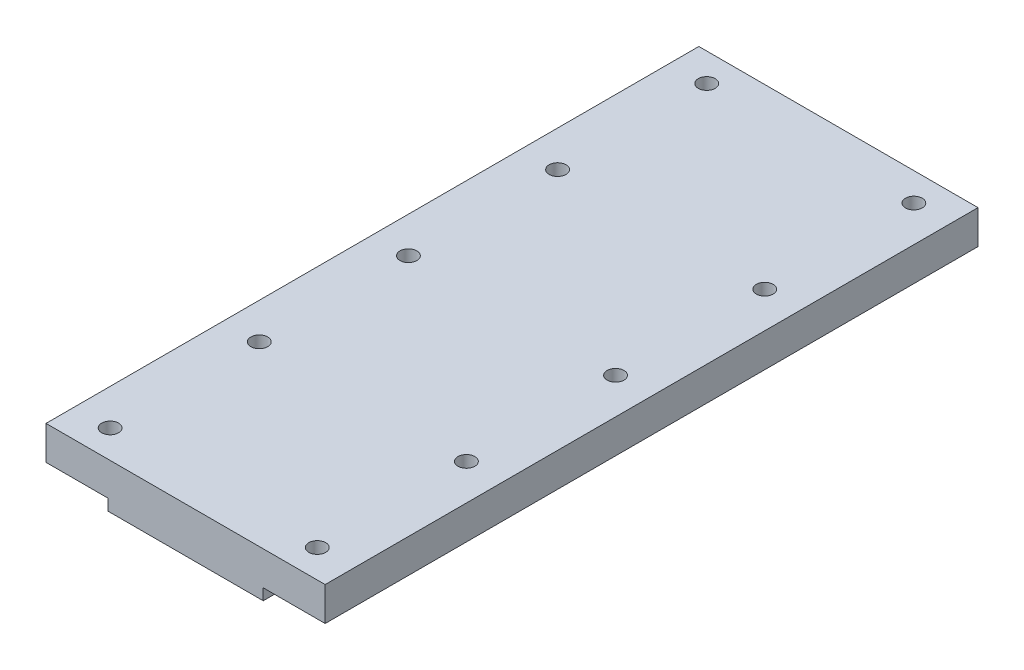
from build123d import *

# Parameters (mm, degrees)
BASE_PLATE_DEPTH            = 290
MOUNTING_HOLES_SKETCH_R     = 7.5
MOUNTING_HOLES_10X_15_DEPTH = 290


with BuildPart() as part:
    # Plate Profile Sketch → Base Plate (new, symmetric)
    with BuildSketch(Plane.XY):
        Polygon((-124, 0), (-69, 0), (-69, -10), (69, -10), (69, 0), (124, 0), (124, 30), (-124, 30), align=None)
    extrude(amount=BASE_PLATE_DEPTH, both=True)

    # Mounting Holes Sketch → Mounting Holes 10xØ15 (cut, symmetric)
    with BuildSketch(Plane(origin=(0, 30, 0), x_dir=(1, 0, 0), z_dir=(0, 1, 0))):
        with Locations(Location((-92, 265, 0), (0, 0, 180))):
            Circle(MOUNTING_HOLES_SKETCH_R)
        with Locations(Location((-92, 132.5, 0), (0, 0, 180))):
            Circle(MOUNTING_HOLES_SKETCH_R)
        with Locations(Location((-92, 0, 0), (0, 0, 180))):
            Circle(MOUNTING_HOLES_SKETCH_R)
        with Locations(Location((-92, -132.5, 0), (0, 0, 180))):
            Circle(MOUNTING_HOLES_SKETCH_R)
        with Locations(Location((-92, -265, 0), (0, 0, 180))):
            Circle(MOUNTING_HOLES_SKETCH_R)
        with Locations(Location((92, 132.5, 0), (0, 0, 270))):
            Circle(MOUNTING_HOLES_SKETCH_R)
        with Locations(Location((92, 0, 0), (0, 0, 270))):
            Circle(MOUNTING_HOLES_SKETCH_R)
        with Locations(Location((92, -132.5, 0), (0, 0, 270))):
            Circle(MOUNTING_HOLES_SKETCH_R)
        with Locations(Location((92, -265, 0), (0, 0, 270))):
            Circle(MOUNTING_HOLES_SKETCH_R)
        with Locations(Location((92, 265, 0), (0, 0, 270))):
            Circle(MOUNTING_HOLES_SKETCH_R)
    extrude(amount=MOUNTING_HOLES_10X_15_DEPTH, both=True, mode=Mode.SUBTRACT)


solid = part.part
